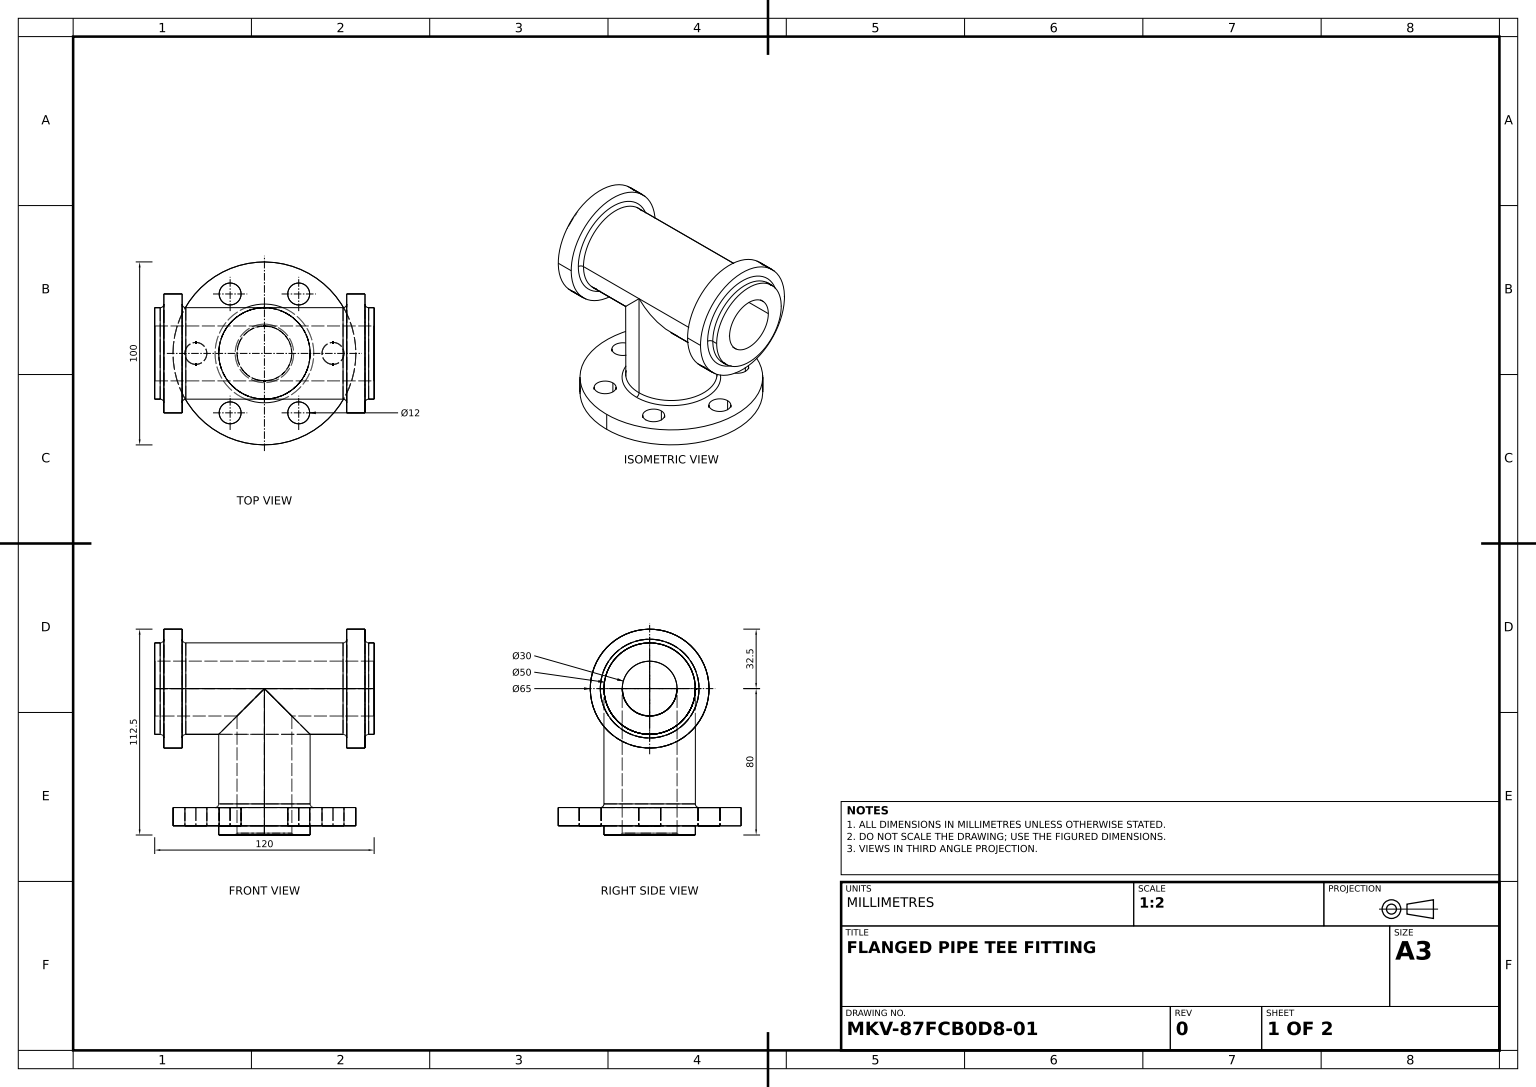
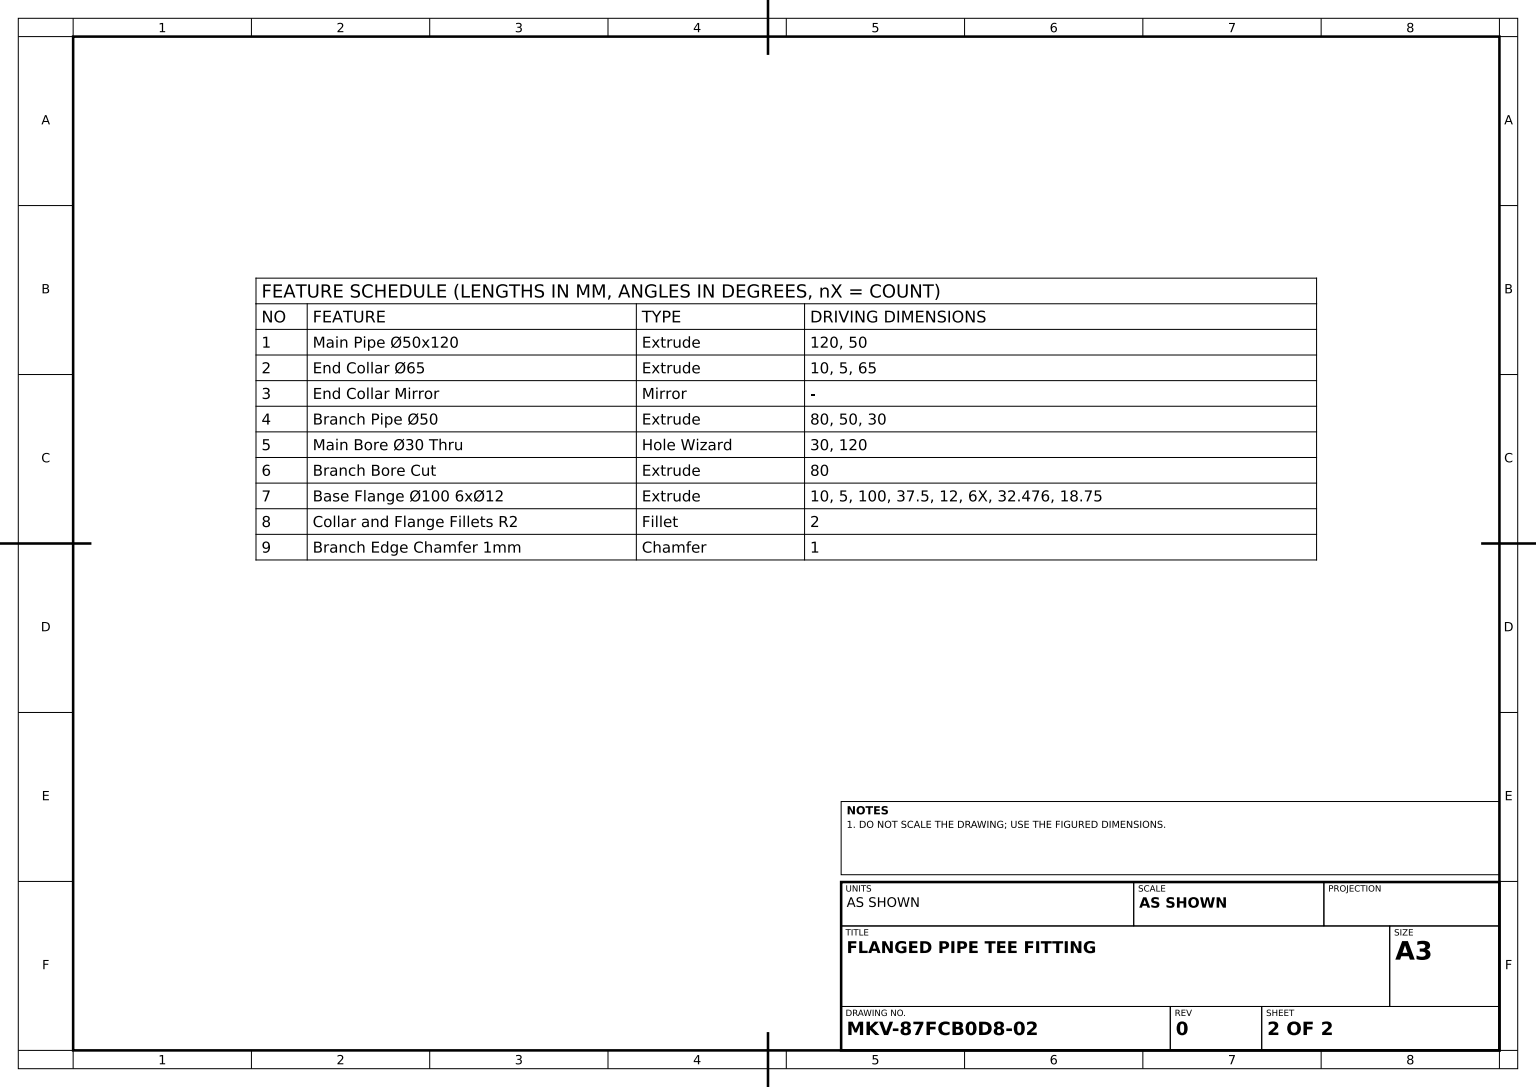
SolidWorks part; units mm, degrees
material "Plain Carbon Steel"
ref_plane "Front Plane" through (0, 0, 0) normal (0, 0, 1) x (1, 0, 0)
ref_plane "Top Plane" through (0, 0, 0) normal (0, 1, 0) x (1, 0, 0)
ref_plane "Right Plane" through (0, 0, 0) normal (1, 0, 0) x (0, 0, -1)
sketch "Main Pipe Sketch" plane through (0, 0, 0) normal (1, 0, 0) x (0, 0, -1)
  circle A0 centre (0, 0) radius 25
  dimension "D1" = 50
extrude "Main Pipe Ø50x120" add sketch "Main Pipe Sketch" along normal mid plane 120
sketch "End Collar Sketch" plane through (60, 0, 0) normal (1, 0, 0) x (0, 0, -1)
  circle A0 centre (0, 0) radius 32.5
  circle A1 centre (0, 0) radius 25 construction
  circle A2 centre (0, 0) radius 25
  dimension "D1" = 65
extrude "End Collar Ø65" add sketch "End Collar Sketch" against normal blind 10 from offset 5 offset against normal yes
mirror "End Collar Mirror" about plane through (0, 0, 0) normal (1, 0, 0) of "End Collar Ø65"
sketch "Branch Pipe Sketch" plane through (0, 0, 0) normal (0, 1, 0) x (1, 0, 0)
  circle A0 centre (0, 0) radius 25
  circle A1 centre (0, 0) radius 15
  dimension "D1" = 50
  dimension "D2" = 30
extrude "Branch Pipe Ø50" add sketch "Branch Pipe Sketch" against normal blind 80
hole_wizard "Main Bore Ø30 Thru" positions "Sketch4" profile "Sketch5" hole size "Ø1.0" standard "ANSI Metric" end condition through all
sketch "Sketch4" plane through (60, 0, 0) normal (1, 0, 0) x (0, 0, -1)
  point P0 (0, 0)
sketch "Sketch5" plane through (60, 0, 0) normal (0, 1, 0) x (0, 0, -1)
  line L0 (0, 0) -> (0, 120)
  line L1 (0, 120) -> (15, 120)
  line L2 (15, 120) -> (15, 0)
  line L5 (15, 0) -> (0, 0)
  line L11 (0, -6.35) -> (0, 107.95) construction
  dimension "Thru Hole Dia." = 30
  dimension "Thru Hole Depth" = 120
sketch "Branch Bore Sketch" plane through (0, 0, 0) normal (0, 1, 0) x (1, 0, 0)
  circle A0 centre (0, 0) radius 15 construction
  circle A1 centre (0, 0) radius 15
extrude "Branch Bore Cut" cut sketch "Branch Bore Sketch" against normal blind 80
sketch "Base Flange Sketch" plane through (0, -80, 0) normal (0, -1, 0) x (1, 0, 0)
  circle A0 centre (0, 0) radius 50
  circle A1 centre (37.5, 0) radius 6
  circle A2 centre (0, 0) radius 25 construction
  circle A3 centre (0, 0) radius 25
  circle A4 centre (18.75, -32.476) radius 6
  circle A5 centre (-18.75, -32.476) radius 6
  circle A6 centre (-37.5, 0) radius 6
  circle A7 centre (-18.75, 32.476) radius 6
  circle A8 centre (18.75, 32.476) radius 6
  point P20 (0, 0)
  dimension "D1" = 100
  dimension "D3" = 12
  dimension "D2" = 37.5
  dimension "D5" = 32.476
  dimension "D6" = 18.75
  dimension "D4" = 6
extrude "Base Flange Ø100 6xØ12" add sketch "Base Flange Sketch" against normal blind 10 from offset 5 offset against normal yes
fillet "Collar and Flange Fillets R2" radius 2 5 edges at (0, -65, -25) (55, 0, -25) (45, 0, -25) (-45, 0, 25) (-55, 0, -25)
chamfer "Branch Edge Chamfer 1mm" distance 1 1 edges at (0, -80, 15)
